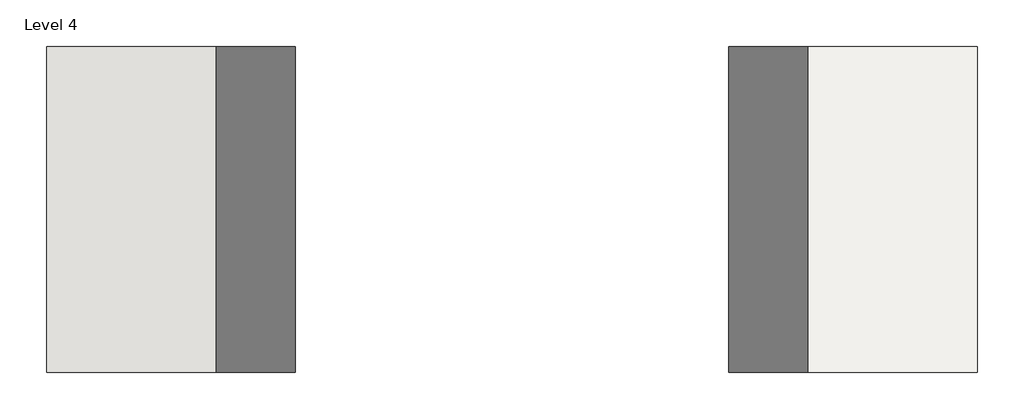
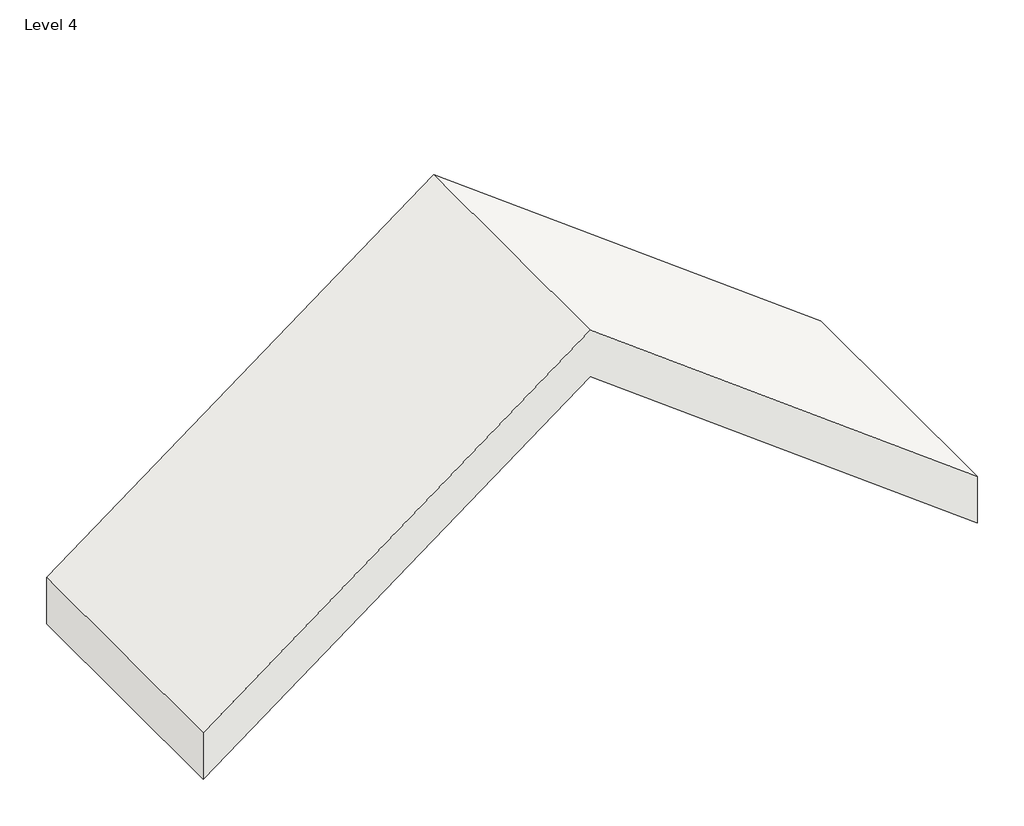
# One storey: 1 roof.
"""IFC4 building model written with IfcOpenShell, lengths in millimetres."""

from ifc_helpers import new_model, si_unit, frame, origin, place, context, project, spatial, polyline, outline, extrude, element, save

model = new_model("IFC4")

# Units and contexts
model_context = context("Model", 3, world=origin())
ifc_project = project(units=[si_unit("LENGTHUNIT", "METRE", prefix="MILLI")], contexts=[model_context])

# Site, building, storey
site = spatial("IfcSite", under=ifc_project)
building = spatial("IfcBuilding", under=site)
storey = spatial("IfcBuildingStorey", under=building, Name="Level 4", Elevation=9144.0)

# Roof
placement = place(None, origin())
element("IfcRoof", 1, ObjectType="Generic - 12\"", at=placement, inside=storey, context=model_context, shape_type="SweptSolid", body=[
    extrude(outline(polyline([(9525.0, -5192.2840012), (11768.8134045, -8184.0352072), (9525.0, -11175.7864131), (9144.0, -11175.7864131), (11387.8134045, -8184.0352072), (9144.0, -5192.2840012), (9525.0, -5192.2840012)])), frame((0.0, -15471.2678064, 0.0), z_axis=(0.0, 1.0, 0.0), x_axis=(0.0, 0.0, 1.0)), (0.0, 0.0, 1.0), 2095.5),
])

save(model, "model.ifc")

# Revit data of these elements
# Type "Generic - 12\""
#   Assembly Code = "B1020"
#   Layers, outside or top first: 1' - 0" no material (function 1)
# Element 1 (IfcRoof, "Generic - 12\"")
#   built-in parameter 1001705 = 38.6116 (stored number, unit not read)
#   built-in parameter 1001710 = 33615
#   Phase Created = New Construction
#   Materials on its faces: "Default Roof"
# Materials
#   "Default Roof": colour RGB 88 101 114, transparency 0, Cost = 0
